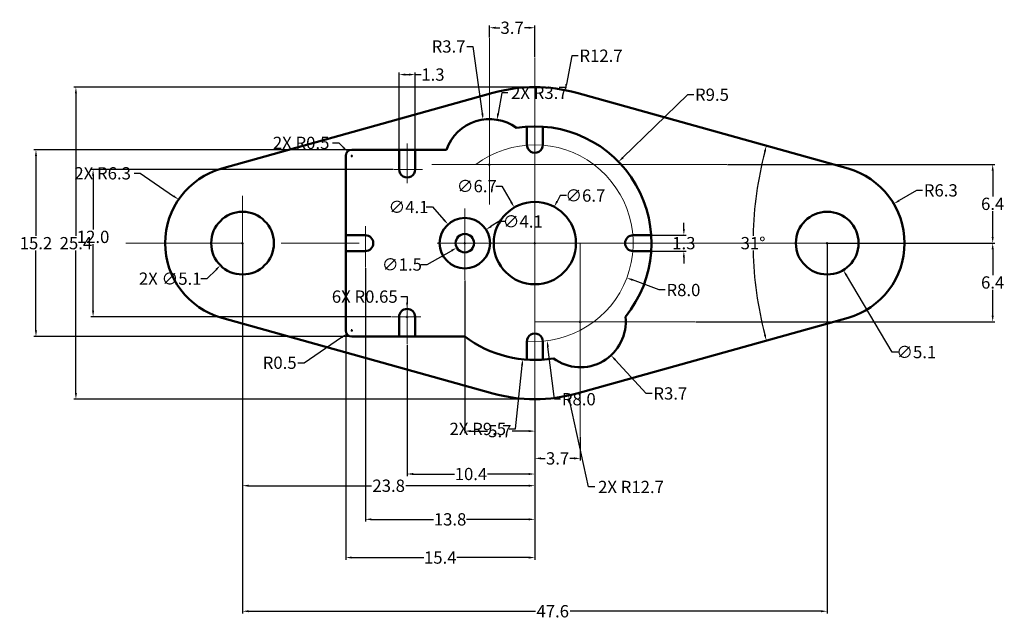
# Model space of a CAD drawing. Units: inches. Extents: x 30.1 to 110.3, y 27.9 to 76.7.
import ezdxf

# ---------------------------------------------------------------- set-up
doc = ezdxf.new("R2010")
doc.units = ezdxf.units.IN
doc.header["$MEASUREMENT"] = 0
doc.linetypes.add('CENTER', pattern=[50.8, 31.75, -6.35, 6.35, -6.35])
for name, color, linetype, lineweight in [('M-CNTR', 4, 'CENTER', 18), ('M-DIMS', 2, 'Continuous', 25), ('M-OUTL', 7, 'Continuous', 50)]:
    doc.layers.add(name, color=color, linetype=linetype, lineweight=lineweight)
doc.styles.get("Standard").update_dxf_attribs({"font": 'arial.ttf'})
doc.dimstyles.get("Standard").update_dxf_attribs({"dimtxt": 1, "dimasz": 0.5, "dimexe": 0.18, "dimexo": 0.0625, "dimgap": 0.09, "dimtad": 0, "dimtih": 1, "dimtoh": 1, "dimdec": 1, "dimzin": 0, "dimdsep": 46, "dimtxsty": 'Standard', "dimcen": 0.09, "dimclrd": 1, "dimclre": 1, "dimadec": 0, "dimazin": 0, "dimtfac": 1, "dimtdec": 1, "dimtofl": 0, "dimtmove": 0, "dimatfit": 3, "dimfxl": 1, "dimtolj": 1, "dimtzin": 0, "dimarcsym": 0})

# ---------------------------------------------------------------- blocks, each defined once
blk = doc.blocks.new('*D1')
at = {"layer": 'Defpoints', "color": 0, "transparency": 16777216}
for p in [(72.073, 43.561), (75.773, 42.842), (75.773, 41.011)]:
    blk.add_point(p, dxfattribs=at)
at = {"layer": 'M-DIMS', "color": 0, "lineweight": -2, "transparency": 16777216}
for p, q in [((72.073, 43.498), (72.073, 40.831)), ((75.773, 42.78), (75.773, 40.831)), ((72.573, 41.011), (72.923, 41.011)), ((75.273, 41.011), (74.923, 41.011))]:
    blk.add_line(p, q, dxfattribs=at)
at = {"layer": 'M-DIMS', "color": 0, "transparency": 16777216}
for points in [[(72.573, 41.095), (72.573, 40.928), (72.073, 41.011)], [(75.273, 41.095), (75.273, 40.928), (75.773, 41.011)]]:
    blk.add_solid(points, dxfattribs=at)
at = {"layer": 'M-DIMS', "color": 0, "transparency": 16777216, "insert": (73.923, 41.011), "char_height": 1, "attachment_point": 5}
blk.add_mtext('\\A1;3.7', dxfattribs=at)
blk = doc.blocks.new('*D2')
at = {"layer": 'Defpoints', "color": 0, "transparency": 16777216}
for p in [(58.273, 56.554), (72.073, 43.561), (72.073, 36.049)]:
    blk.add_point(p, dxfattribs=at)
at = {"layer": 'M-DIMS', "color": 0, "lineweight": -2, "transparency": 16777216}
for p, q in [((58.273, 56.492), (58.273, 35.869)), ((72.073, 43.498), (72.073, 35.869)), ((58.773, 36.049), (63.83, 36.049)), ((71.573, 36.049), (66.516, 36.049))]:
    blk.add_line(p, q, dxfattribs=at)
at = {"layer": 'M-DIMS', "color": 0, "transparency": 16777216}
for points in [[(58.773, 36.132), (58.773, 35.966), (58.273, 36.049)], [(71.573, 36.132), (71.573, 35.966), (72.073, 36.049)]]:
    blk.add_solid(points, dxfattribs=at)
at = {"layer": 'M-DIMS', "color": 0, "transparency": 16777216, "insert": (65.173, 36.049), "char_height": 1, "attachment_point": 5}
blk.add_mtext('\\A1;13.8', dxfattribs=at)
blk = doc.blocks.new('*D3')
at = {"layer": 'Defpoints', "color": 0, "transparency": 16777216}
for p in [(61.673, 50.328), (72.073, 43.561), (72.073, 39.74)]:
    blk.add_point(p, dxfattribs=at)
at = {"layer": 'M-DIMS', "color": 0, "lineweight": -2, "transparency": 16777216}
for p, q in [((61.673, 50.265), (61.673, 39.56)), ((72.073, 43.498), (72.073, 39.56)), ((62.173, 39.74), (65.533, 39.74)), ((71.573, 39.74), (68.213, 39.74))]:
    blk.add_line(p, q, dxfattribs=at)
at = {"layer": 'M-DIMS', "color": 0, "transparency": 16777216}
for points in [[(62.173, 39.823), (62.173, 39.657), (61.673, 39.74)], [(71.573, 39.823), (71.573, 39.657), (72.073, 39.74)]]:
    blk.add_solid(points, dxfattribs=at)
at = {"layer": 'M-DIMS', "color": 0, "transparency": 16777216, "insert": (66.873, 39.74), "char_height": 1, "attachment_point": 5}
blk.add_mtext('\\A1;10.4', dxfattribs=at)
blk = doc.blocks.new('*D4')
at = {"layer": 'Defpoints', "color": 0, "transparency": 16777216}
for p in [(66.373, 55.542), (72.073, 43.561), (72.073, 43.231)]:
    blk.add_point(p, dxfattribs=at)
at = {"layer": 'M-DIMS', "color": 0, "lineweight": -2, "transparency": 16777216}
for p, q in [((66.373, 55.48), (66.373, 43.051)), ((72.073, 43.498), (72.073, 43.051)), ((66.873, 43.231), (68.223, 43.231)), ((71.573, 43.231), (70.223, 43.231))]:
    blk.add_line(p, q, dxfattribs=at)
at = {"layer": 'M-DIMS', "color": 0, "transparency": 16777216}
for points in [[(66.873, 43.314), (66.873, 43.147), (66.373, 43.231)], [(71.573, 43.314), (71.573, 43.147), (72.073, 43.231)]]:
    blk.add_solid(points, dxfattribs=at)
at = {"layer": 'M-DIMS', "color": 0, "transparency": 16777216, "insert": (69.223, 43.231), "char_height": 1, "attachment_point": 5}
blk.add_mtext('\\A1;5.7', dxfattribs=at)
blk = doc.blocks.new('*D5')
at = {"layer": 'Defpoints', "color": 0, "transparency": 16777216}
for p in [(48.273, 58.527), (95.873, 58.527), (95.873, 28.571)]:
    blk.add_point(p, dxfattribs=at)
at = {"layer": 'M-DIMS', "color": 0, "lineweight": -2, "transparency": 16777216}
for p, q in [((48.273, 58.465), (48.273, 28.391)), ((95.873, 58.465), (95.873, 28.391)), ((48.773, 28.571), (72.121, 28.571)), ((95.373, 28.571), (74.938, 28.571))]:
    blk.add_line(p, q, dxfattribs=at)
at = {"layer": 'M-DIMS', "color": 0, "transparency": 16777216}
for points in [[(48.773, 28.655), (48.773, 28.488), (48.273, 28.571)], [(95.373, 28.655), (95.373, 28.488), (95.873, 28.571)]]:
    blk.add_solid(points, dxfattribs=at)
at = {"layer": 'M-DIMS', "color": 0, "transparency": 16777216, "insert": (73.529, 28.571), "char_height": 1, "attachment_point": 5}
blk.add_mtext('\\A1;47.6', dxfattribs=at)
blk = doc.blocks.new('*D6')
at = {"layer": 'Defpoints', "color": 0, "transparency": 16777216}
for p in [(60.6, 64.527), (36.108, 52.527), (60.401, 52.527)]:
    blk.add_point(p, dxfattribs=at)
at = {"layer": 'M-DIMS', "color": 0, "lineweight": -2, "transparency": 16777216}
for p, q in [((60.538, 64.527), (35.928, 64.527)), ((36.108, 64.027), (36.108, 59.638)), ((36.108, 53.027), (36.108, 58.437)), ((60.338, 52.527), (35.928, 52.527))]:
    blk.add_line(p, q, dxfattribs=at)
at = {"layer": 'M-DIMS', "color": 0, "transparency": 16777216}
for points in [[(36.025, 64.027), (36.191, 64.027), (36.108, 64.527)], [(36.025, 53.027), (36.191, 53.027), (36.108, 52.527)]]:
    blk.add_solid(points, dxfattribs=at)
at = {"layer": 'M-DIMS', "color": 0, "transparency": 16777216, "insert": (36.108, 59.038), "char_height": 1, "attachment_point": 5}
blk.add_mtext('\\A1;12.0', dxfattribs=at)
blk = doc.blocks.new('*D7')
at = {"layer": 'Defpoints', "color": 0, "transparency": 16777216}
for p in [(75.773, 52.127), (78.275, 49.401)]:
    blk.add_point(p, dxfattribs=at)
at = {"layer": 'M-DIMS', "color": 0, "lineweight": -2, "transparency": 16777216}
for p, q in [((75.683, 52.127), (75.863, 52.127)), ((75.773, 52.037), (75.773, 52.217)), ((81.124, 46.295), (78.613, 49.033)), ((81.624, 46.295), (81.124, 46.295))]:
    blk.add_line(p, q, dxfattribs=at)
at = {"layer": 'M-DIMS', "color": 0, "transparency": 16777216}
blk.add_solid([(78.674, 49.089), (78.551, 48.976), (78.275, 49.401)], dxfattribs=at)
at = {"layer": 'M-DIMS', "color": 0, "transparency": 16777216, "insert": (83.103, 46.295), "char_height": 1, "attachment_point": 5}
blk.add_mtext('\\A1;R3.7', dxfattribs=at)
blk = doc.blocks.new('*D8')
at = {"layer": 'Defpoints', "color": 0, "transparency": 16777216}
for p in [(72.073, 58.527), (79.559, 55.707)]:
    blk.add_point(p, dxfattribs=at)
at = {"layer": 'M-DIMS', "color": 0, "lineweight": -2, "transparency": 16777216}
for p, q in [((71.983, 58.527), (72.163, 58.527)), ((72.073, 58.437), (72.073, 58.617)), ((82.193, 54.715), (80.027, 55.531)), ((82.693, 54.715), (82.193, 54.715))]:
    blk.add_line(p, q, dxfattribs=at)
at = {"layer": 'M-DIMS', "color": 0, "transparency": 16777216}
blk.add_solid([(80.057, 55.609), (79.998, 55.453), (79.559, 55.707)], dxfattribs=at)
at = {"layer": 'M-DIMS', "color": 0, "transparency": 16777216, "insert": (84.17, 54.715), "char_height": 1, "attachment_point": 5}
blk.add_mtext('\\A1;R8.0', dxfattribs=at)
blk = doc.blocks.new('*D9')
at = {"layer": 'Defpoints', "color": 0, "transparency": 16777216}
for p in [(81.551, 59.177), (81.551, 57.877), (84.204, 57.877)]:
    blk.add_point(p, dxfattribs=at)
at = {"layer": 'M-DIMS', "color": 0, "lineweight": -2, "transparency": 16777216}
for p, q in [((84.204, 59.677), (84.204, 60.177)), ((81.613, 59.177), (84.384, 59.177)), ((81.613, 57.877), (84.384, 57.877)), ((84.204, 57.377), (84.204, 56.877))]:
    blk.add_line(p, q, dxfattribs=at)
at = {"layer": 'M-DIMS', "color": 0, "transparency": 16777216}
for points in [[(84.121, 59.677), (84.288, 59.677), (84.204, 59.177)], [(84.121, 57.377), (84.288, 57.377), (84.204, 57.877)]]:
    blk.add_solid(points, dxfattribs=at)
at = {"layer": 'M-DIMS', "color": 0, "transparency": 16777216, "insert": (84.204, 58.527), "char_height": 1, "attachment_point": 5}
blk.add_mtext('\\A1;1.3', dxfattribs=at)
blk = doc.blocks.new('*D10')
at = {"layer": 'Defpoints', "color": 0, "transparency": 16777216}
for p in [(73.648, 61.484), (70.498, 55.57)]:
    blk.add_point(p, dxfattribs=at)
at = {"layer": 'M-DIMS', "color": 0, "lineweight": -2, "transparency": 16777216}
for p, q in [((74.137, 62.402), (73.883, 61.925)), ((74.637, 62.402), (74.137, 62.402)), ((71.983, 58.527), (72.163, 58.527)), ((72.073, 58.437), (72.073, 58.617))]:
    blk.add_line(p, q, dxfattribs=at)
at = {"layer": 'M-DIMS', "color": 0, "transparency": 16777216}
blk.add_solid([(73.809, 61.965), (73.956, 61.886), (73.648, 61.484)], dxfattribs=at)
at = {"layer": 'M-DIMS', "color": 0, "transparency": 16777216, "insert": (76.181, 62.402), "char_height": 1, "attachment_point": 5}
blk.add_mtext('\\A1;∅6.7', dxfattribs=at)
blk = doc.blocks.new('*D11')
at = {"layer": 'Defpoints', "color": 0, "transparency": 16777216}
for p in [(65.006, 60.054), (67.741, 57)]:
    blk.add_point(p, dxfattribs=at)
at = {"layer": 'M-DIMS', "color": 0, "lineweight": -2, "transparency": 16777216}
for p, q in [((63.237, 61.471), (63.737, 61.471)), ((63.737, 61.471), (64.672, 60.427)), ((66.283, 58.527), (66.463, 58.527)), ((66.373, 58.437), (66.373, 58.617))]:
    blk.add_line(p, q, dxfattribs=at)
at = {"layer": 'M-DIMS', "color": 0, "transparency": 16777216}
blk.add_solid([(64.734, 60.483), (64.61, 60.371), (65.006, 60.054)], dxfattribs=at)
at = {"layer": 'M-DIMS', "color": 0, "transparency": 16777216, "insert": (61.789, 61.471), "char_height": 1, "attachment_point": 5}
blk.add_mtext('\\A1;∅4.1', dxfattribs=at)
blk = doc.blocks.new('*D12')
at = {"layer": 'Defpoints', "color": 0, "transparency": 16777216}
for p in [(67.026, 58.896), (65.72, 58.158)]:
    blk.add_point(p, dxfattribs=at)
at = {"layer": 'M-DIMS', "color": 0, "lineweight": -2, "transparency": 16777216}
for p, q in [((66.283, 58.527), (66.463, 58.527)), ((66.373, 58.437), (66.373, 58.617)), ((63.298, 56.79), (65.285, 57.912)), ((62.798, 56.79), (63.298, 56.79))]:
    blk.add_line(p, q, dxfattribs=at)
at = {"layer": 'M-DIMS', "color": 0, "transparency": 16777216}
blk.add_solid([(65.244, 57.985), (65.326, 57.84), (65.72, 58.158)], dxfattribs=at)
at = {"layer": 'M-DIMS', "color": 0, "transparency": 16777216, "insert": (61.25, 56.79), "char_height": 1, "attachment_point": 5}
blk.add_mtext('\\A1;∅1.5', dxfattribs=at)
blk = doc.blocks.new('*D13')
at = {"layer": 'Defpoints', "color": 0, "transparency": 16777216}
for p in [(62.323, 72.246), (61.023, 66.127), (62.323, 66.127)]:
    blk.add_point(p, dxfattribs=at)
at = {"layer": 'M-DIMS', "color": 0, "lineweight": -2, "transparency": 16777216}
for p, q in [((61.023, 66.19), (61.023, 72.426)), ((61.523, 72.246), (61.823, 72.246)), ((62.323, 66.19), (62.323, 72.426)), ((62.323, 72.246), (62.823, 72.246))]:
    blk.add_line(p, q, dxfattribs=at)
at = {"layer": 'M-DIMS', "color": 0, "transparency": 16777216}
for points in [[(61.523, 72.329), (61.523, 72.162), (61.023, 72.246)], [(61.823, 72.329), (61.823, 72.162), (62.323, 72.246)]]:
    blk.add_solid(points, dxfattribs=at)
at = {"layer": 'M-DIMS', "color": 0, "transparency": 16777216, "insert": (63.776, 72.246), "char_height": 1, "attachment_point": 5}
blk.add_mtext('\\A1;1.3', dxfattribs=at)
blk = doc.blocks.new('*D14')
at = {"layer": 'Defpoints', "color": 0, "transparency": 16777216}
for p in [(67.86, 68.592), (68.373, 64.927)]:
    blk.add_point(p, dxfattribs=at)
at = {"layer": 'M-DIMS', "color": 0, "lineweight": -2, "transparency": 16777216}
for p, q in [((66.528, 74.533), (67.028, 74.533)), ((67.028, 74.533), (67.791, 69.087)), ((68.373, 64.837), (68.373, 65.017)), ((68.283, 64.927), (68.463, 64.927))]:
    blk.add_line(p, q, dxfattribs=at)
at = {"layer": 'M-DIMS', "color": 0, "transparency": 16777216}
blk.add_solid([(67.873, 69.098), (67.708, 69.075), (67.86, 68.592)], dxfattribs=at)
at = {"layer": 'M-DIMS', "color": 0, "transparency": 16777216, "insert": (65.049, 74.533), "char_height": 1, "attachment_point": 5}
blk.add_mtext('\\A1;R3.7', dxfattribs=at)
blk = doc.blocks.new('*D15')
at = {"layer": 'Defpoints', "color": 0, "transparency": 16777216}
for p in [(72.073, 76.057), (68.373, 75.206), (72.073, 73.633)]:
    blk.add_point(p, dxfattribs=at)
at = {"layer": 'M-DIMS', "color": 0, "lineweight": -2, "transparency": 16777216}
for p, q in [((68.373, 75.269), (68.373, 76.237)), ((72.073, 73.695), (72.073, 76.237)), ((68.873, 76.057), (69.223, 76.057)), ((71.573, 76.057), (71.223, 76.057))]:
    blk.add_line(p, q, dxfattribs=at)
at = {"layer": 'M-DIMS', "color": 0, "transparency": 16777216}
for points in [[(68.873, 76.14), (68.873, 75.974), (68.373, 76.057)], [(71.573, 76.14), (71.573, 75.974), (72.073, 76.057)]]:
    blk.add_solid(points, dxfattribs=at)
at = {"layer": 'M-DIMS', "color": 0, "transparency": 16777216, "insert": (70.223, 76.057), "char_height": 1, "attachment_point": 5}
blk.add_mtext('\\A1;3.7', dxfattribs=at)
blk = doc.blocks.new('*D16')
at = {"layer": 'Defpoints', "color": 0, "transparency": 16777216}
for p in [(74.54, 70.985), (72.073, 58.527)]:
    blk.add_point(p, dxfattribs=at)
at = {"layer": 'M-DIMS', "color": 0, "lineweight": -2, "transparency": 16777216}
for p, q in [((75.093, 73.782), (74.637, 71.476)), ((75.593, 73.782), (75.093, 73.782)), ((71.983, 58.527), (72.163, 58.527)), ((72.073, 58.437), (72.073, 58.617))]:
    blk.add_line(p, q, dxfattribs=at)
at = {"layer": 'M-DIMS', "color": 0, "transparency": 16777216}
blk.add_solid([(74.555, 71.492), (74.719, 71.46), (74.54, 70.985)], dxfattribs=at)
at = {"layer": 'M-DIMS', "color": 0, "transparency": 16777216, "insert": (77.461, 73.782), "char_height": 1, "attachment_point": 5}
blk.add_mtext('\\A1;R12.7', dxfattribs=at)
blk = doc.blocks.new('*D17')
at = {"layer": 'Defpoints', "color": 0, "transparency": 16777216}
for p in [(78.886, 65.148), (72.073, 58.527)]:
    blk.add_point(p, dxfattribs=at)
at = {"layer": 'M-DIMS', "color": 0, "lineweight": -2, "transparency": 16777216}
for p, q in [((84.509, 70.611), (79.245, 65.496)), ((85.009, 70.611), (84.509, 70.611)), ((71.983, 58.527), (72.163, 58.527)), ((72.073, 58.437), (72.073, 58.617))]:
    blk.add_line(p, q, dxfattribs=at)
at = {"layer": 'M-DIMS', "color": 0, "transparency": 16777216}
blk.add_solid([(79.187, 65.556), (79.303, 65.436), (78.886, 65.148)], dxfattribs=at)
at = {"layer": 'M-DIMS', "color": 0, "transparency": 16777216, "insert": (86.492, 70.611), "char_height": 1, "attachment_point": 5}
blk.add_mtext('\\A1;R9.5', dxfattribs=at)
blk = doc.blocks.new('*D18')
at = {"layer": 'Defpoints', "color": 0, "transparency": 16777216}
for p in [(75.488, 70.759), (97.567, 64.595), (89.958, 61.198), (97.567, 52.459), (75.488, 46.295)]:
    blk.add_point(p, dxfattribs=at)
at = {"layer": 'M-DIMS', "color": 0, "lineweight": -2, "transparency": 16777216}
for start, end in [(165.37302, 178.83141), (181.16859, 194.62698)]:
    blk.add_arc((119.301, 58.527), 29.465, start, end, dxfattribs=at)
at = {"layer": 'M-DIMS', "color": 0, "transparency": 16777216}
for points in [[(90.711, 65.99), (90.872, 65.946), (90.922, 66.451)], [(90.872, 51.108), (90.711, 51.065), (90.922, 50.604)]]:
    blk.add_solid(points, dxfattribs=at)
at = {"layer": 'M-DIMS', "color": 0, "transparency": 16777216, "insert": (89.837, 58.527), "char_height": 1, "attachment_point": 5}
blk.add_mtext('\\A1;31°', dxfattribs=at)
blk = doc.blocks.new('*D19')
at = {"layer": 'Defpoints', "color": 0, "transparency": 16777216}
for p in [(101.297, 61.733), (95.873, 58.527)]:
    blk.add_point(p, dxfattribs=at)
at = {"layer": 'M-DIMS', "color": 0, "lineweight": -2, "transparency": 16777216}
for p, q in [((103.142, 62.823), (101.727, 61.987)), ((103.642, 62.823), (103.142, 62.823)), ((95.783, 58.527), (95.963, 58.527)), ((95.873, 58.437), (95.873, 58.617))]:
    blk.add_line(p, q, dxfattribs=at)
at = {"layer": 'M-DIMS', "color": 0, "transparency": 16777216}
blk.add_solid([(101.685, 62.059), (101.769, 61.915), (101.297, 61.733)], dxfattribs=at)
at = {"layer": 'M-DIMS', "color": 0, "transparency": 16777216, "insert": (105.12, 62.823), "char_height": 1, "attachment_point": 5}
blk.add_mtext('\\A1;R6.3', dxfattribs=at)
blk = doc.blocks.new('*D20')
at = {"layer": 'Defpoints', "color": 0, "transparency": 16777216}
for p in [(94.564, 60.716), (97.182, 56.339)]:
    blk.add_point(p, dxfattribs=at)
at = {"layer": 'M-DIMS', "color": 0, "lineweight": -2, "transparency": 16777216}
for p, q in [((95.783, 58.527), (95.963, 58.527)), ((95.873, 58.437), (95.873, 58.617)), ((101.175, 49.663), (97.439, 55.91)), ((101.675, 49.663), (101.175, 49.663))]:
    blk.add_line(p, q, dxfattribs=at)
at = {"layer": 'M-DIMS', "color": 0, "transparency": 16777216}
blk.add_solid([(97.51, 55.953), (97.367, 55.867), (97.182, 56.339)], dxfattribs=at)
at = {"layer": 'M-DIMS', "color": 0, "transparency": 16777216, "insert": (103.123, 49.663), "char_height": 1, "attachment_point": 5}
blk.add_mtext('\\A1;∅5.1', dxfattribs=at)
blk = doc.blocks.new('*D21')
at = {"layer": 'Defpoints', "color": 0, "transparency": 16777216}
for p in [(87.707, 64.927), (102.173, 58.527), (109.345, 58.527)]:
    blk.add_point(p, dxfattribs=at)
at = {"layer": 'M-DIMS', "color": 0, "lineweight": -2, "transparency": 16777216}
for p, q in [((87.77, 64.927), (109.525, 64.927)), ((109.345, 64.427), (109.345, 62.328)), ((109.345, 59.027), (109.345, 61.127)), ((102.236, 58.527), (109.525, 58.527))]:
    blk.add_line(p, q, dxfattribs=at)
at = {"layer": 'M-DIMS', "color": 0, "transparency": 16777216}
for points in [[(109.262, 64.427), (109.429, 64.427), (109.345, 64.927)], [(109.262, 59.027), (109.429, 59.027), (109.345, 58.527)]]:
    blk.add_solid(points, dxfattribs=at)
at = {"layer": 'M-DIMS', "color": 0, "transparency": 16777216, "insert": (109.345, 61.727), "char_height": 1, "attachment_point": 5}
blk.add_mtext('\\A1;6.4', dxfattribs=at)
blk = doc.blocks.new('*D22')
at = {"layer": 'Defpoints', "color": 0, "transparency": 16777216}
for p in [(95.783, 58.527), (109.345, 58.527), (85.114, 52.127)]:
    blk.add_point(p, dxfattribs=at)
at = {"layer": 'M-DIMS', "color": 0, "lineweight": -2, "transparency": 16777216}
for p, q in [((95.846, 58.527), (109.525, 58.527)), ((109.345, 58.027), (109.345, 55.928)), ((109.345, 52.627), (109.345, 54.727)), ((85.176, 52.127), (109.525, 52.127))]:
    blk.add_line(p, q, dxfattribs=at)
at = {"layer": 'M-DIMS', "color": 0, "transparency": 16777216}
for points in [[(109.262, 58.027), (109.429, 58.027), (109.345, 58.527)], [(109.262, 52.627), (109.429, 52.627), (109.345, 52.127)]]:
    blk.add_solid(points, dxfattribs=at)
at = {"layer": 'M-DIMS', "color": 0, "transparency": 16777216, "insert": (109.345, 55.327), "char_height": 1, "attachment_point": 5}
blk.add_mtext('\\A1;6.4', dxfattribs=at)
blk = doc.blocks.new('*D23')
at = {"layer": 'Defpoints', "color": 0, "transparency": 16777216}
for p in [(57.173, 51.427), (56.759, 51.147)]:
    blk.add_point(p, dxfattribs=at)
at = {"layer": 'M-DIMS', "color": 0, "lineweight": -2, "transparency": 16777216}
for p, q in [((57.083, 51.427), (57.263, 51.427)), ((57.173, 51.337), (57.173, 51.517)), ((53.281, 48.795), (56.345, 50.867)), ((52.781, 48.795), (53.281, 48.795))]:
    blk.add_line(p, q, dxfattribs=at)
at = {"layer": 'M-DIMS', "color": 0, "transparency": 16777216}
blk.add_solid([(56.298, 50.936), (56.391, 50.798), (56.759, 51.147)], dxfattribs=at)
at = {"layer": 'M-DIMS', "color": 0, "transparency": 16777216, "insert": (51.298, 48.795), "char_height": 1, "attachment_point": 5}
blk.add_mtext('\\A1;R0.5', dxfattribs=at)
blk = doc.blocks.new('*D24')
at = {"layer": 'Defpoints', "color": 0, "transparency": 16777216}
for p in [(56.673, 51.427), (72.073, 43.561), (72.073, 32.94)]:
    blk.add_point(p, dxfattribs=at)
at = {"layer": 'M-DIMS', "color": 0, "lineweight": -2, "transparency": 16777216}
for p, q in [((56.673, 51.365), (56.673, 32.76)), ((72.073, 43.498), (72.073, 32.76)), ((57.173, 32.94), (63.033, 32.94)), ((71.573, 32.94), (65.713, 32.94))]:
    blk.add_line(p, q, dxfattribs=at)
at = {"layer": 'M-DIMS', "color": 0, "transparency": 16777216}
for points in [[(57.173, 33.024), (57.173, 32.857), (56.673, 32.94)], [(71.573, 33.024), (71.573, 32.857), (72.073, 32.94)]]:
    blk.add_solid(points, dxfattribs=at)
at = {"layer": 'M-DIMS', "color": 0, "transparency": 16777216, "insert": (64.373, 32.94), "char_height": 1, "attachment_point": 5}
blk.add_mtext('\\A1;15.4', dxfattribs=at)
blk = doc.blocks.new('*D25')
at = {"layer": 'Defpoints', "color": 0, "transparency": 16777216}
for p in [(57.173, 66.127), (31.459, 50.927), (57.173, 50.927)]:
    blk.add_point(p, dxfattribs=at)
at = {"layer": 'M-DIMS', "color": 0, "lineweight": -2, "transparency": 16777216}
for p, q in [((57.111, 66.127), (31.279, 66.127)), ((31.459, 65.627), (31.459, 59.128)), ((31.459, 51.427), (31.459, 57.927)), ((57.111, 50.927), (31.279, 50.927))]:
    blk.add_line(p, q, dxfattribs=at)
at = {"layer": 'M-DIMS', "color": 0, "transparency": 16777216}
for points in [[(31.375, 65.627), (31.542, 65.627), (31.459, 66.127)], [(31.375, 51.427), (31.542, 51.427), (31.459, 50.927)]]:
    blk.add_solid(points, dxfattribs=at)
at = {"layer": 'M-DIMS', "color": 0, "transparency": 16777216, "insert": (31.459, 58.527), "char_height": 1, "attachment_point": 5}
blk.add_mtext('\\A1;15.2', dxfattribs=at)
blk = doc.blocks.new('FLANGE-MOUNTING-EAR')
blk.add_circle((6.3, 6.068), 2.55)
blk.add_arc((6.3, 6.068), 6.3, 105.59927, 254.40073)
blk = doc.blocks.new('ALIGNMENT-SLOT-1_3')
for p, q in [((1.6, 1.3), (0, 1.3)), ((0, 1.3), (0, 0)), ((1.6, 0), (0, 0))]:
    blk.add_line(p, q)
blk.add_arc((1.6, 0.65), 0.65, 270, 90)
blk = doc.blocks.new('HUB-ALIGNMENT-NOTCH')
for p, q in [((0.001, 0.624), (0.001, 2.128)), ((1.3, 0.65), (1.3, 2.128))]:
    blk.add_line(p, q)
blk.add_arc((0.65, 0.65), 0.65, 177.67172, 0)
blk = doc.blocks.new('*D29')
at = {"layer": 'Defpoints', "color": 0, "transparency": 16777216}
for p in [(34.71, 71.227), (72.073, 71.227), (72.073, 45.827)]:
    blk.add_point(p, dxfattribs=at)
at = {"layer": 'M-DIMS', "color": 1, "lineweight": -2, "transparency": 16777216}
for p, q in [((72.011, 71.227), (34.53, 71.227)), ((34.71, 70.727), (34.71, 59.128)), ((34.71, 46.327), (34.71, 57.927)), ((72.011, 45.827), (34.53, 45.827))]:
    blk.add_line(p, q, dxfattribs=at)
at = {"layer": 'M-DIMS', "color": 1, "transparency": 16777216}
for points in [[(34.627, 70.727), (34.793, 70.727), (34.71, 71.227)], [(34.627, 46.327), (34.793, 46.327), (34.71, 45.827)]]:
    blk.add_solid(points, dxfattribs=at)
at = {"layer": 'M-DIMS', "color": 0, "transparency": 16777216, "insert": (34.71, 58.527), "char_height": 1, "attachment_point": 5}
blk.add_mtext('\\A1;25.4', dxfattribs=at)
blk = doc.blocks.new('*D30')
at = {"layer": 'Defpoints', "color": 0, "transparency": 16777216}
for p in [(48.273, 55.977), (72.073, 45.827), (72.073, 38.787)]:
    blk.add_point(p, dxfattribs=at)
at = {"layer": 'M-DIMS', "color": 1, "lineweight": -2, "transparency": 16777216}
for p, q in [((48.273, 55.915), (48.273, 38.607)), ((72.073, 45.765), (72.073, 38.607)), ((48.773, 38.787), (58.775, 38.787)), ((71.573, 38.787), (61.571, 38.787))]:
    blk.add_line(p, q, dxfattribs=at)
at = {"layer": 'M-DIMS', "color": 1, "transparency": 16777216}
for points in [[(48.773, 38.871), (48.773, 38.704), (48.273, 38.787)], [(71.573, 38.871), (71.573, 38.704), (72.073, 38.787)]]:
    blk.add_solid(points, dxfattribs=at)
at = {"layer": 'M-DIMS', "color": 0, "transparency": 16777216, "insert": (60.173, 38.787), "char_height": 1, "attachment_point": 5}
blk.add_mtext('\\A1;23.8', dxfattribs=at)
blk = doc.blocks.new('*D31')
at = {"layer": 'Defpoints', "color": 0, "transparency": 16777216}
for p in [(72.073, 58.527), (74.81, 46.126)]:
    blk.add_point(p, dxfattribs=at)
at = {"layer": 'M-DIMS', "color": 1, "lineweight": -2, "transparency": 16777216}
for p, q in [((71.983, 58.527), (72.163, 58.527)), ((72.073, 58.437), (72.073, 58.617)), ((76.452, 38.685), (74.918, 45.637)), ((76.952, 38.685), (76.452, 38.685))]:
    blk.add_line(p, q, dxfattribs=at)
at = {"layer": 'M-DIMS', "color": 1, "transparency": 16777216}
blk.add_solid([(74.999, 45.655), (74.836, 45.619), (74.81, 46.126)], dxfattribs=at)
at = {"layer": 'M-DIMS', "color": 0, "transparency": 16777216, "insert": (79.902, 38.685), "char_height": 1, "attachment_point": 5}
blk.add_mtext('\\A1;2X R12.7', dxfattribs=at)
blk = doc.blocks.new('*D32')
at = {"layer": 'Defpoints', "color": 0, "transparency": 16777216}
for p in [(72.073, 58.527), (71.085, 49.079)]:
    blk.add_point(p, dxfattribs=at)
at = {"layer": 'M-DIMS', "color": 1, "lineweight": -2, "transparency": 16777216}
for p, q in [((71.983, 58.527), (72.163, 58.527)), ((72.073, 58.437), (72.073, 58.617)), ((70.492, 43.41), (71.033, 48.582)), ((69.992, 43.41), (70.492, 43.41))]:
    blk.add_line(p, q, dxfattribs=at)
at = {"layer": 'M-DIMS', "color": 1, "transparency": 16777216}
blk.add_solid([(70.95, 48.59), (71.116, 48.573), (71.085, 49.079)], dxfattribs=at)
at = {"layer": 'M-DIMS', "color": 0, "transparency": 16777216, "insert": (67.427, 43.41), "char_height": 1, "attachment_point": 5}
blk.add_mtext('\\A1;2X R9.5', dxfattribs=at)
blk = doc.blocks.new('*D33')
at = {"layer": 'Defpoints', "color": 0, "transparency": 16777216}
for p in [(72.073, 58.527), (73.073, 50.59)]:
    blk.add_point(p, dxfattribs=at)
at = {"layer": 'M-DIMS', "color": 1, "lineweight": -2, "transparency": 16777216}
for p, q in [((71.983, 58.527), (72.163, 58.527)), ((72.073, 58.437), (72.073, 58.617)), ((73.673, 45.828), (73.135, 50.094)), ((74.173, 45.828), (73.673, 45.828))]:
    blk.add_line(p, q, dxfattribs=at)
at = {"layer": 'M-DIMS', "color": 1, "transparency": 16777216}
blk.add_solid([(73.218, 50.104), (73.053, 50.084), (73.073, 50.59)], dxfattribs=at)
at = {"layer": 'M-DIMS', "color": 0, "transparency": 16777216, "insert": (75.65, 45.828), "char_height": 1, "attachment_point": 5}
blk.add_mtext('\\A1;R8.0', dxfattribs=at)
blk = doc.blocks.new('*D34')
at = {"layer": 'Defpoints', "color": 0, "transparency": 16777216}
for p in [(43.07, 62.08), (48.273, 58.527)]:
    blk.add_point(p, dxfattribs=at)
at = {"layer": 'M-DIMS', "color": 1, "lineweight": -2, "transparency": 16777216}
for p, q in [((39.449, 64.211), (39.949, 64.211)), ((39.949, 64.211), (42.657, 62.362)), ((48.183, 58.527), (48.363, 58.527)), ((48.273, 58.437), (48.273, 58.617))]:
    blk.add_line(p, q, dxfattribs=at)
at = {"layer": 'M-DIMS', "color": 1, "transparency": 16777216}
blk.add_solid([(42.704, 62.431), (42.61, 62.293), (43.07, 62.08)], dxfattribs=at)
at = {"layer": 'M-DIMS', "color": 0, "transparency": 16777216, "insert": (36.887, 64.211), "char_height": 1, "attachment_point": 5}
blk.add_mtext('\\A1;2X R6.3', dxfattribs=at)
blk = doc.blocks.new('*D35')
at = {"layer": 'Defpoints', "color": 0, "transparency": 16777216}
for p in [(69, 68.574), (68.373, 64.927)]:
    blk.add_point(p, dxfattribs=at)
at = {"layer": 'M-DIMS', "color": 1, "lineweight": -2, "transparency": 16777216}
for p, q in [((69.376, 70.762), (69.085, 69.067)), ((69.876, 70.762), (69.376, 70.762)), ((68.373, 64.837), (68.373, 65.017)), ((68.283, 64.927), (68.463, 64.927))]:
    blk.add_line(p, q, dxfattribs=at)
at = {"layer": 'M-DIMS', "color": 1, "transparency": 16777216}
blk.add_solid([(69.003, 69.081), (69.167, 69.052), (69, 68.574)], dxfattribs=at)
at = {"layer": 'M-DIMS', "color": 0, "transparency": 16777216, "insert": (72.438, 70.762), "char_height": 1, "attachment_point": 5}
blk.add_mtext('\\A1;2X R3.7', dxfattribs=at)
blk = doc.blocks.new('*D36')
at = {"layer": 'Defpoints', "color": 0, "transparency": 16777216}
for p in [(70.398, 61.428), (73.748, 55.626)]:
    blk.add_point(p, dxfattribs=at)
at = {"layer": 'M-DIMS', "color": 1, "lineweight": -2, "transparency": 16777216}
for p, q in [((68.893, 63.169), (69.393, 63.169)), ((69.393, 63.169), (70.148, 61.861)), ((71.983, 58.527), (72.163, 58.527)), ((72.073, 58.437), (72.073, 58.617))]:
    blk.add_line(p, q, dxfattribs=at)
at = {"layer": 'M-DIMS', "color": 1, "transparency": 16777216}
blk.add_solid([(70.22, 61.903), (70.076, 61.82), (70.398, 61.428)], dxfattribs=at)
at = {"layer": 'M-DIMS', "color": 0, "transparency": 16777216, "insert": (67.348, 63.169), "char_height": 1, "attachment_point": 5}
blk.add_mtext('\\A1;∅6.7', dxfattribs=at)
blk = doc.blocks.new('*D37')
at = {"layer": 'Defpoints', "color": 0, "transparency": 16777216}
for p in [(50.074, 60.333), (46.472, 56.722)]:
    blk.add_point(p, dxfattribs=at)
at = {"layer": 'M-DIMS', "color": 1, "lineweight": -2, "transparency": 16777216}
for p, q in [((48.183, 58.527), (48.363, 58.527)), ((48.273, 58.437), (48.273, 58.617)), ((45.391, 55.639), (46.119, 56.368)), ((44.891, 55.639), (45.391, 55.639))]:
    blk.add_line(p, q, dxfattribs=at)
at = {"layer": 'M-DIMS', "color": 1, "transparency": 16777216}
blk.add_solid([(46.06, 56.427), (46.178, 56.309), (46.472, 56.722)], dxfattribs=at)
at = {"layer": 'M-DIMS', "color": 0, "transparency": 16777216, "insert": (42.387, 55.639), "char_height": 1, "attachment_point": 5}
blk.add_mtext('\\A1;2X ∅5.1', dxfattribs=at)
blk = doc.blocks.new('*D38')
at = {"layer": 'Defpoints', "color": 0, "transparency": 16777216}
for p in [(68.102, 59.629), (64.644, 57.425)]:
    blk.add_point(p, dxfattribs=at)
at = {"layer": 'M-DIMS', "color": 1, "lineweight": -2, "transparency": 16777216}
for p, q in [((69.139, 60.29), (68.523, 59.898)), ((69.639, 60.29), (69.139, 60.29)), ((66.283, 58.527), (66.463, 58.527)), ((66.373, 58.437), (66.373, 58.617))]:
    blk.add_line(p, q, dxfattribs=at)
at = {"layer": 'M-DIMS', "color": 1, "transparency": 16777216}
blk.add_solid([(68.479, 59.968), (68.568, 59.828), (68.102, 59.629)], dxfattribs=at)
at = {"layer": 'M-DIMS', "color": 0, "transparency": 16777216, "insert": (71.087, 60.29), "char_height": 1, "attachment_point": 5}
blk.add_mtext('\\A1;∅4.1', dxfattribs=at)
blk = doc.blocks.new('*D39')
at = {"layer": 'Defpoints', "color": 0, "transparency": 16777216}
for p in [(61.673, 53.177), (61.673, 52.527)]:
    blk.add_point(p, dxfattribs=at)
at = {"layer": 'M-DIMS', "color": 1, "lineweight": -2, "transparency": 16777216}
for p, q in [((61.173, 54.177), (61.673, 54.177)), ((61.673, 54.177), (61.673, 53.677)), ((61.583, 52.527), (61.763, 52.527)), ((61.673, 52.437), (61.673, 52.617))]:
    blk.add_line(p, q, dxfattribs=at)
at = {"layer": 'M-DIMS', "color": 1, "transparency": 16777216}
blk.add_solid([(61.756, 53.677), (61.59, 53.677), (61.673, 53.177)], dxfattribs=at)
at = {"layer": 'M-DIMS', "color": 0, "transparency": 16777216, "insert": (58.225, 54.177), "char_height": 1, "attachment_point": 5}
blk.add_mtext('\\A1;6X R0.65', dxfattribs=at)
blk = doc.blocks.new('*D40')
at = {"layer": 'Defpoints', "color": 0, "transparency": 16777216}
for p in [(56.819, 65.981), (57.173, 65.627)]:
    blk.add_point(p, dxfattribs=at)
at = {"layer": 'M-DIMS', "color": 1, "lineweight": -2, "transparency": 16777216}
for p, q in [((55.612, 66.687), (56.112, 66.687)), ((56.112, 66.687), (56.466, 66.334)), ((57.083, 65.627), (57.263, 65.627)), ((57.173, 65.537), (57.173, 65.717))]:
    blk.add_line(p, q, dxfattribs=at)
at = {"layer": 'M-DIMS', "color": 1, "transparency": 16777216}
blk.add_solid([(56.525, 66.393), (56.407, 66.275), (56.819, 65.981)], dxfattribs=at)
at = {"layer": 'M-DIMS', "color": 0, "transparency": 16777216, "insert": (53.046, 66.687), "char_height": 1, "attachment_point": 5}
blk.add_mtext('\\A1;2X R0.5', dxfattribs=at)

msp = doc.modelspace()

# ---------------------------------------------------------------- linework, layer by layer
at = {"layer": 'M-CNTR'}
for p, q in [((68.373, 61.682), (68.373, 75.206)), ((72.073, 73.633), (72.073, 43.561)), ((61.673, 63.408), (61.673, 66.63)), ((60.6, 64.527), (62.936, 64.527)), ((87.707, 64.927), (63.686, 64.927)), ((48.273, 62.38), (48.273, 54.443)), ((66.373, 61.356), (66.373, 55.542)), ((58.273, 59.907), (58.273, 56.554)), ((68.373, 58.527), (68.373, 58.977)), ((75.773, 58.527), (75.773, 42.842)), ((61.673, 53.942), (61.673, 50.328)), ((60.401, 52.527), (62.786, 52.527)), ((72.073, 52.127), (85.114, 52.127))]:
    msp.add_line(p, q, dxfattribs=at)
msp.add_lwpolyline([(95.873, 58.527), (48.273, 58.527), (38.765, 58.527)], dxfattribs=at)
msp.add_arc((72.073, 58.527), 8, 265.34344, 126.8699, dxfattribs=at)
at = {"layer": 'M-OUTL'}
for p, q in [((46.579, 64.595), (68.658, 70.759)), ((97.567, 64.595), (75.488, 70.759)), ((57.173, 66.127), (61.023, 66.127)), ((62.323, 66.127), (64.873, 66.127)), ((56.673, 59.177), (56.673, 65.627)), ((80.073, 59.177), (81.551, 59.177)), ((56.673, 57.877), (56.673, 51.427)), ((80.073, 57.877), (81.551, 57.877)), ((46.579, 52.459), (68.658, 46.295)), ((97.567, 52.459), (75.488, 46.295)), ((57.173, 50.927), (61.023, 50.927)), ((62.323, 50.927), (66.373, 50.927))]:
    msp.add_line(p, q, dxfattribs=at)
for centre, radius in [((72.073, 58.527), 3.35), ((66.373, 58.527), 2.05), ((66.373, 58.527), 0.75)]:
    msp.add_circle(centre, radius, dxfattribs=at)
for centre, radius, start, end in [((72.073, 58.527), 12.7, 74.40073, 105.59927), ((68.373, 64.927), 3.7, 53.64347, 161.07536), ((72.073, 58.527), 9.5, 320.94146, 99.1251), ((57.173, 65.627), 0.5, 90, 180), ((80.073, 58.527), 0.65, 90, 270), ((75.773, 52.127), 3.7, 233.64347, 6.42309), ((57.173, 51.427), 0.5, 180, 270), ((72.073, 58.527), 9.5, 233.1301, 279.1251), ((72.073, 58.527), 12.7, 254.40073, 285.59927)]:
    msp.add_arc(centre, radius, start, end, dxfattribs=at)

# ---------------------------------------------------------------- block references
for name, p in [('HUB-ALIGNMENT-NOTCH', (71.423, 65.877)), ('FLANGE-MOUNTING-EAR', (41.973, 52.459)), ('ALIGNMENT-SLOT-1_3', (56.673, 57.877))]:
    msp.add_blockref(name, p, dxfattribs=at)
for name, p, rotation in [('ALIGNMENT-SLOT-1_3', (61.023, 66.127), 270.0000000000001), ('FLANGE-MOUNTING-EAR', (102.173, 64.596), 180), ('ALIGNMENT-SLOT-1_3', (62.323, 50.927), 90.00000000000053)]:
    msp.add_blockref(name, p, dxfattribs=dict(at, rotation=rotation))
at = {"layer": 'M-OUTL', "extrusion": (0, 0, -1), "zscale": -1, "rotation": 180}
msp.add_blockref('HUB-ALIGNMENT-NOTCH', (-71.423, 51.178), dxfattribs=at)

# ---------------------------------------------------------------- dimensions: what is measured, and where the dimension line sits
at = {"layer": 'M-DIMS'}
for base, p1, p2, override, picture, middle in [((72.073, 76.057), (68.373, 75.206), (72.073, 73.633), {"dimclrd": 0, "dimclre": 0, "dimclrt": 0}, '*D15', (70.223, 76.057)), ((62.323, 72.246), (61.023, 66.127), (62.323, 66.127), {"dimclrd": 0, "dimclre": 0, "dimclrt": 0}, '*D13', (63.776, 72.246)), ((72.073, 38.787), (48.273, 55.977), (72.073, 45.827), {"dimdec": 1, "dimlfac": 1, "dimrnd": 0, "dimzin": 0, "dimdsep": 46, "dimlunit": 2}, '*D30', (60.173, 38.787)), ((72.073, 43.231), (66.373, 55.542), (72.073, 43.561), {"dimclrd": 0, "dimclre": 0, "dimclrt": 0}, '*D4', (69.223, 43.231)), ((72.073, 32.94), (56.673, 51.427), (72.073, 43.561), {"dimclrd": 0, "dimclre": 0, "dimclrt": 0}, '*D24', (64.373, 32.94)), ((72.073, 39.74), (61.673, 50.328), (72.073, 43.561), {"dimclrd": 0, "dimclre": 0, "dimclrt": 0}, '*D3', (66.873, 39.74)), ((75.773, 41.011), (72.073, 43.561), (75.773, 42.842), {"dimclrd": 0, "dimclre": 0, "dimclrt": 0}, '*D1', (73.923, 41.011))]:
    dim = msp.add_linear_dim(base=base, p1=p1, p2=p2, dimstyle='Standard', override=override, dxfattribs=at)
    dim.commit()
    dim.dimension.update_dxf_attribs({"geometry": picture, "text_midpoint": middle})
for center, mpoint, override, picture, middle in [((68.373, 64.927), (67.86, 68.592), {"dimclrd": 0, "dimclre": 0, "dimclrt": 0}, '*D14', (65.049, 74.533)), ((72.073, 58.527), (74.54, 70.985), {"dimclrd": 0, "dimclre": 0, "dimclrt": 0}, '*D16', (77.461, 73.782)), ((72.073, 58.527), (78.886, 65.148), {"dimclrd": 0, "dimclre": 0, "dimclrt": 0}, '*D17', (86.492, 70.611)), ((95.873, 58.527), (101.297, 61.733), {"dimclrd": 0, "dimclre": 0, "dimclrt": 0}, '*D19', (105.12, 62.823)), ((72.073, 58.527), (79.559, 55.707), {"dimclrd": 0, "dimclre": 0, "dimclrt": 0}, '*D8', (84.17, 54.715)), ((72.073, 58.527), (73.073, 50.59), {"dimdec": 1, "dimlfac": 1, "dimrnd": 0, "dimzin": 0, "dimdsep": 46, "dimlunit": 2}, '*D33', (75.65, 45.828)), ((75.773, 52.127), (78.275, 49.401), {"dimclrd": 0, "dimclre": 0, "dimclrt": 0}, '*D7', (83.103, 46.295)), ((57.173, 51.427), (56.759, 51.147), {"dimclrd": 0, "dimclre": 0, "dimclrt": 0}, '*D23', (51.298, 48.795))]:
    dim = msp.add_radius_dim(center=center, mpoint=mpoint, dimstyle='Standard', override=override, dxfattribs=at)
    dim.commit()
    dim.dimension.update_dxf_attribs({"geometry": picture, "text_midpoint": middle, "dimtype": 164})
for center, mpoint, picture, middle in [((68.373, 64.927), (69, 68.574), '*D35', (72.438, 70.762)), ((48.273, 58.527), (43.07, 62.08), '*D34', (36.887, 64.211)), ((72.073, 58.527), (71.085, 49.079), '*D32', (67.427, 43.41)), ((72.073, 58.527), (74.81, 46.126), '*D31', (79.902, 38.685))]:
    dim = msp.add_radius_dim(center=center, mpoint=mpoint, text='2X <>', dimstyle='Standard', override={"dimdec": 1, "dimlfac": 1, "dimrnd": 0, "dimzin": 0, "dimdsep": 46, "dimlunit": 2}, dxfattribs=at)
    dim.commit()
    dim.dimension.update_dxf_attribs({"geometry": picture, "text_midpoint": middle, "dimtype": 164})
for base, p1, p2, override, picture, middle in [((34.71, 71.227), (72.073, 45.827), (72.073, 71.227), {"dimdec": 1, "dimlfac": 1, "dimrnd": 0, "dimzin": 0, "dimdsep": 46, "dimlunit": 2}, '*D29', (34.71, 58.527)), ((31.459, 50.927), (57.173, 66.127), (57.173, 50.927), {"dimclrd": 0, "dimclre": 0, "dimclrt": 0}, '*D25', (31.459, 58.527)), ((84.204, 57.877), (81.551, 59.177), (81.551, 57.877), {"dimclrd": 0, "dimclre": 0, "dimclrt": 0}, '*D9', (84.204, 58.527)), ((109.345, 58.527), (85.114, 52.127), (95.783, 58.527), {"dimclrd": 0, "dimclre": 0, "dimclrt": 0}, '*D22', (109.345, 55.327))]:
    dim = msp.add_linear_dim(base=base, p1=p1, p2=p2, angle=90, dimstyle='Standard', override=override, dxfattribs=at)
    dim.commit()
    dim.dimension.update_dxf_attribs({"geometry": picture, "text_midpoint": middle})
dim = msp.add_angular_dim_2l(base=(89.958, 61.198), line1=((97.567, 52.459), (75.488, 46.295)), line2=((97.567, 64.595), (75.488, 70.759)), dimstyle='Standard', override={"dimclrd": 0, "dimclre": 0, "dimclrt": 0}, dxfattribs=at)
dim.commit()
dim.dimension.update_dxf_attribs({"geometry": '*D18', "text_midpoint": (89.837, 58.527)})
for center, mpoint, text, override, picture, middle in [((57.173, 65.627), (56.819, 65.981), '2X <>', {"dimdec": 1, "dimlfac": 1, "dimrnd": 0, "dimzin": 0, "dimdsep": 46, "dimlunit": 2}, '*D40', (53.046, 66.687)), ((61.673, 52.527), (61.673, 53.177), '6X <>', {"dimdec": 2, "dimlfac": 1, "dimrnd": 0, "dimzin": 0, "dimdsep": 46, "dimlunit": 2}, '*D39', (58.225, 54.177))]:
    dim = msp.add_radius_dim(center=center, mpoint=mpoint, text=text, dimstyle='Standard', override=override, dxfattribs=at)
    dim.commit()
    dim.dimension.update_dxf_attribs({"geometry": picture, "text_midpoint": middle})
for base, p1, p2, picture, middle in [((36.108, 52.527), (60.6, 64.527), (60.401, 52.527), '*D6', (36.108, 59.038)), ((109.345, 58.527), (87.707, 64.927), (102.173, 58.527), '*D21', (109.345, 61.727))]:
    dim = msp.add_linear_dim(base=base, p1=p1, p2=p2, angle=90, dimstyle='Standard', override={"dimclrd": 0, "dimclre": 0, "dimclrt": 0}, dxfattribs=at)
    dim.commit()
    dim.dimension.update_dxf_attribs({"geometry": picture, "text_midpoint": middle, "dimtype": 160})
for p1, p2, override, picture, middle in [((73.748, 55.626), (70.398, 61.428), {"dimdec": 1, "dimlfac": 1, "dimrnd": 0, "dimzin": 0, "dimdsep": 46, "dimlunit": 2}, '*D36', (67.348, 63.169)), ((70.498, 55.57), (73.648, 61.484), {"dimclrd": 0, "dimclre": 0, "dimclrt": 0}, '*D10', (76.181, 62.402)), ((67.741, 57), (65.006, 60.054), {"dimclrd": 0, "dimclre": 0, "dimclrt": 0}, '*D11', (61.789, 61.471)), ((64.644, 57.425), (68.102, 59.629), {"dimdec": 1, "dimlfac": 1, "dimrnd": 0, "dimzin": 0, "dimdsep": 46, "dimlunit": 2}, '*D38', (71.087, 60.29)), ((94.564, 60.716), (97.182, 56.339), {"dimclrd": 0, "dimclre": 0, "dimclrt": 0}, '*D20', (103.123, 49.663)), ((67.026, 58.896), (65.72, 58.158), {"dimclrd": 0, "dimclre": 0, "dimclrt": 0}, '*D12', (61.25, 56.79))]:
    dim = msp.add_diameter_dim_2p(p1=p1, p2=p2, dimstyle='Standard', override=override, dxfattribs=at)
    dim.commit()
    dim.dimension.update_dxf_attribs({"geometry": picture, "text_midpoint": middle, "dimtype": 163})
dim = msp.add_diameter_dim_2p(p1=(50.074, 60.333), p2=(46.472, 56.722), text='2X <>', dimstyle='Standard', override={"dimdec": 1, "dimlfac": 1, "dimrnd": 0, "dimzin": 0, "dimdsep": 46, "dimlunit": 2}, dxfattribs=at)
dim.commit()
dim.dimension.update_dxf_attribs({"geometry": '*D37', "text_midpoint": (42.387, 55.639), "dimtype": 163})
for base, p1, p2, picture, middle in [((95.873, 28.571), (48.273, 58.527), (95.873, 58.527), '*D5', (73.529, 28.571)), ((72.073, 36.049), (58.273, 56.554), (72.073, 43.561), '*D2', (65.173, 36.049))]:
    dim = msp.add_linear_dim(base=base, p1=p1, p2=p2, dimstyle='Standard', override={"dimclrd": 0, "dimclre": 0, "dimclrt": 0}, dxfattribs=at)
    dim.commit()
    dim.dimension.update_dxf_attribs({"geometry": picture, "text_midpoint": middle, "dimtype": 160})

doc.saveas('drawing.dxf')
